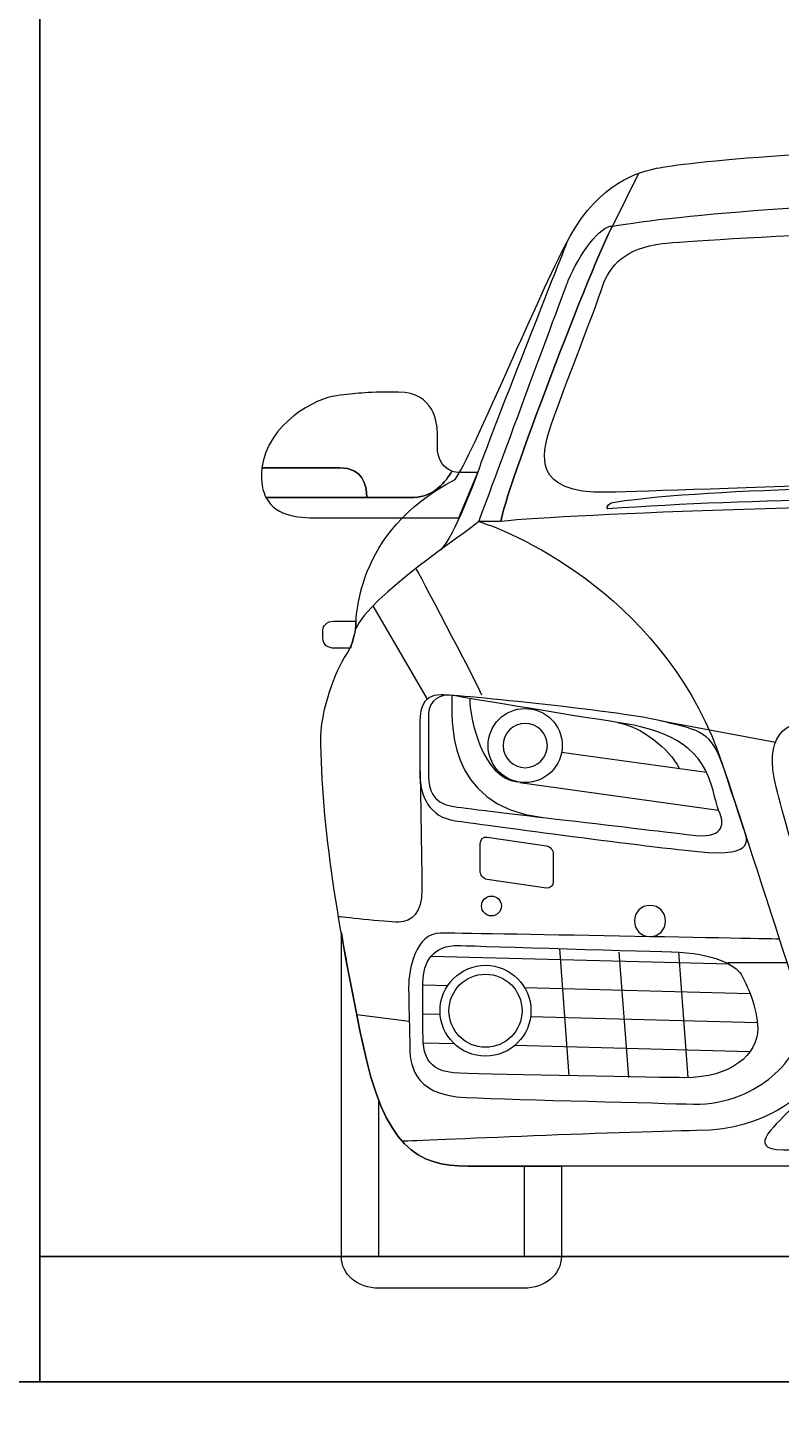
# Model space of a CAD drawing. Units: inches. Extents: x 1152 to 2588, y 1459 to 2618.
# Tile 9 of 17: x 1285 to 1321, y 2319 to 2386. Entities that reach past the tile are written whole.
import ezdxf

# ---------------------------------------------------------------- set-up
doc = ezdxf.new("R2010")
doc.units = ezdxf.units.IN
for name, color, linetype, lineweight in [('A-ANNO-DIMS', 2, 'Continuous', 18), ('A-ELEV', 7, 'Continuous', 25), ('AUDI', 7, 'Continuous', 13)]:
    doc.layers.add(name, color=color, linetype=linetype, lineweight=lineweight)
doc.styles.get("Standard").update_dxf_attribs({"font": 'arial.ttf'})
doc.dimstyles.get("Standard").update_dxf_attribs({"dimtxt": 0.18, "dimasz": 0.18, "dimexe": 0.18, "dimexo": 0.0625, "dimgap": 0.09, "dimtad": 0, "dimtih": 1, "dimtoh": 1, "dimdec": 4, "dimzin": 0, "dimdsep": 46, "dimtxsty": 'Standard', "dimcen": 0.09, "dimadec": 0, "dimazin": 0, "dimtfac": 1, "dimtdec": 4, "dimtofl": 0, "dimtmove": 0, "dimatfit": 3, "dimfxl": 1, "dimtolj": 1, "dimtzin": 0, "dimarcsym": 0})

# ---------------------------------------------------------------- blocks, each defined once
blk = doc.blocks.new('*D91')
at = {"layer": 'A-ANNO-DIMS', "color": 0, "lineweight": -2, "transparency": 16777216}
for p, q in [((1405.417, 2327.329), (1405.417, 2232.94)), ((1276.417, 2321.329), (1276.417, 2232.94)), ((1276.597, 2233.12), (1340.636, 2233.12)), ((1405.237, 2233.12), (1341.197, 2233.12))]:
    blk.add_line(p, q, dxfattribs=at)
at = {"layer": 'A-ANNO-DIMS', "color": 0, "transparency": 16777216}
for points in [[(1276.597, 2233.15), (1276.597, 2233.09), (1276.417, 2233.12)], [(1405.237, 2233.15), (1405.237, 2233.09), (1405.417, 2233.12)]]:
    blk.add_solid(points, dxfattribs=at)
at = {"layer": 'Defpoints', "color": 0, "transparency": 16777216}
for p in [(1405.417, 2327.391), (1276.417, 2321.391), (1405.417, 2233.12)]:
    blk.add_point(p, dxfattribs=at)
at = {"layer": 'A-ANNO-DIMS', "color": 0, "transparency": 16777216, "insert": (1340.917, 2233.12), "char_height": 0.18, "attachment_point": 5}
blk.add_mtext('\\A1;129', dxfattribs=at)

msp = doc.modelspace()

# ---------------------------------------------------------------- linework, layer by layer
at = {"layer": 'A-ELEV'}
for p, q in [((1285.4165, 2453.3911), (1285.4165, 2327.3911)), ((1736.4165, 2327.3911), (1285.4165, 2327.3911)), ((1285.4165, 2327.3911), (1285.4165, 2321.3911)), ((1736.4165, 2321.3911), (1276.4165, 2321.3911))]:
    msp.add_line(p, q, dxfattribs=at)
at = {"layer": 'AUDI'}
for points, knots in [([(1335.9514, 2380.6082), (1323.07, 2380.6082), (1316.2344, 2379.8209), (1314.9649, 2379.5565), (1314.9649, 2379.5565), (1313.6952, 2379.292), (1311.974, 2378.5979), (1310.5458, 2375.7943), (1310.5458, 2375.7943), (1309.1176, 2372.9909), (1306.1088, 2365.771), (1305.3217, 2364.6395), (1305.3217, 2364.6395), (1300.4024, 2362.1057), (1300.5918, 2357.8087), (1300.5428, 2357.4642), (1300.5428, 2357.4642), (1300.4936, 2357.1198), (1300.2995, 2356.5002), (1300.0824, 2356.2017), (1300.0824, 2356.2017), (1299.5785, 2355.5088), (1298.8858, 2353.5262), (1298.8858, 2352.3397), (1298.8858, 2352.3397), (1298.8858, 2347.9967), (1299.7554, 2343.0506), (1300.8566, 2337.73), (1300.8566, 2337.73), (1301.9224, 2332.5811), (1303.5104, 2331.7248), (1305.9177, 2331.7248), (1305.9177, 2331.7248), (1307.7191, 2331.725), (1335.9514, 2331.7248), (1335.9514, 2331.7248), (1335.9514, 2331.7248), (1335.9514, 2331.725), (1364.1837, 2331.7248), (1365.9852, 2331.7248), (1365.9852, 2331.7248), (1368.3925, 2331.725), (1369.9807, 2332.581), (1371.0466, 2337.73), (1371.0466, 2337.73), (1372.1483, 2343.0506), (1373.0181, 2347.9966), (1373.0181, 2352.3397), (1373.0181, 2352.3397), (1373.0181, 2353.5264), (1372.3251, 2355.5087), (1371.8212, 2356.2017), (1371.8212, 2356.2017), (1371.6039, 2356.5003), (1371.41, 2357.1198), (1371.3608, 2357.4642), (1371.3608, 2357.4642), (1371.3116, 2357.8087), (1371.501, 2362.1057), (1366.5811, 2364.6395), (1366.5811, 2364.6395), (1365.7941, 2365.7711), (1362.7853, 2372.9908), (1361.357, 2375.7943), (1361.357, 2375.7943), (1359.9288, 2378.5979), (1358.2076, 2379.292), (1356.9379, 2379.5565), (1356.9379, 2379.5565), (1355.6684, 2379.821), (1348.8329, 2380.608), (1335.9514, 2380.6082)], [0, 0, 0, 0, 0.0555556, 0.0555556, 0.0555556, 0.0555556, 0.1111111, 0.1111111, 0.1111111, 0.1111111, 0.1666667, 0.1666667, 0.1666667, 0.1666667, 0.2222222, 0.2222222, 0.2222222, 0.2222222, 0.2777778, 0.2777778, 0.2777778, 0.2777778, 0.3333333, 0.3333333, 0.3333333, 0.3333333, 0.3888889, 0.3888889, 0.3888889, 0.3888889, 0.4444444, 0.4444444, 0.4444444, 0.4444445, 0.5, 0.5, 0.5, 0.5, 0.5555556, 0.5555556, 0.5555556, 0.5555556, 0.6111111, 0.6111111, 0.6111111, 0.6111111, 0.6666667, 0.6666667, 0.6666667, 0.6666667, 0.7222222, 0.7222222, 0.7222222, 0.7222222, 0.7777778, 0.7777778, 0.7777778, 0.7777778, 0.8333333, 0.8333333, 0.8333333, 0.8333333, 0.8888889, 0.8888889, 0.8888889, 0.8888889, 0.9444444, 0.9444444, 0.9444444, 0.9444445, 1, 1, 1, 1]), ([(1335.9514, 2380.6082), (1323.07, 2380.6082), (1316.2344, 2379.8209), (1314.9649, 2379.5565), (1314.9649, 2379.5565), (1313.6952, 2379.292), (1311.974, 2378.5979), (1310.5458, 2375.7943), (1310.5458, 2375.7943), (1309.1176, 2372.9909), (1306.1088, 2365.771), (1305.3217, 2364.6395), (1305.3217, 2364.6395), (1300.4024, 2362.1057), (1300.5918, 2357.8087), (1300.5428, 2357.4642), (1300.5428, 2357.4642), (1300.4936, 2357.1198), (1300.2995, 2356.5002), (1300.0824, 2356.2017), (1300.0824, 2356.2017), (1299.5785, 2355.5088), (1298.8858, 2353.5262), (1298.8858, 2352.3397), (1298.8858, 2352.3397), (1298.8858, 2347.9967), (1299.7554, 2343.0506), (1300.8566, 2337.73), (1300.8566, 2337.73), (1301.9224, 2332.5811), (1303.5104, 2331.7248), (1305.9177, 2331.7248), (1305.9177, 2331.7248), (1307.7191, 2331.725), (1335.9514, 2331.7248), (1335.9514, 2331.7248), (1335.9514, 2331.7248), (1335.9514, 2331.7248), (1364.1837, 2331.7248), (1365.9852, 2331.7248), (1365.9852, 2331.7248), (1368.3925, 2331.725), (1369.9807, 2332.581), (1371.0466, 2337.73), (1371.0466, 2337.73), (1372.1483, 2343.0506), (1373.0181, 2347.9966), (1373.0181, 2352.3397), (1373.0181, 2352.3397), (1373.0181, 2353.5264), (1372.3251, 2355.5087), (1371.8212, 2356.2017), (1371.8212, 2356.2017), (1371.6039, 2356.5003), (1371.41, 2357.1198), (1371.3608, 2357.4642), (1371.3608, 2357.4642), (1371.3116, 2357.8087), (1371.501, 2362.1057), (1366.5811, 2364.6395), (1366.5811, 2364.6395), (1365.7941, 2365.7711), (1362.7853, 2372.9908), (1361.357, 2375.7943), (1361.357, 2375.7943), (1359.9288, 2378.5979), (1358.2076, 2379.292), (1356.9379, 2379.5565), (1356.9379, 2379.5565), (1355.6684, 2379.821), (1348.8329, 2380.608), (1335.9514, 2380.6082)], [0, 0, 0, 0, 0.0555556, 0.0555556, 0.0555556, 0.0555556, 0.1111111, 0.1111111, 0.1111111, 0.1111111, 0.1666667, 0.1666667, 0.1666667, 0.1666667, 0.2222222, 0.2222222, 0.2222222, 0.2222222, 0.2777778, 0.2777778, 0.2777778, 0.2777778, 0.3333333, 0.3333333, 0.3333333, 0.3333333, 0.3888889, 0.3888889, 0.3888889, 0.3888889, 0.4444444, 0.4444444, 0.4444444, 0.4444445, 0.5, 0.5, 0.5, 0.5, 0.5555556, 0.5555556, 0.5555556, 0.5555556, 0.6111111, 0.6111111, 0.6111111, 0.6111111, 0.6666667, 0.6666667, 0.6666667, 0.6666667, 0.7222222, 0.7222222, 0.7222222, 0.7222222, 0.7777778, 0.7777778, 0.7777778, 0.7777778, 0.8333333, 0.8333333, 0.8333333, 0.8333333, 0.8888889, 0.8888889, 0.8888889, 0.8888889, 0.9444444, 0.9444444, 0.9444444, 0.9444445, 1, 1, 1, 1]), ([(1335.9514, 2378.0831), (1323.862, 2378.0831), (1315.9013, 2377.3042), (1312.8453, 2376.7794), (1312.8453, 2376.7794), (1311.9763, 2375.2275), (1307.631, 2363.8673), (1307.5068, 2362.6256), (1307.5068, 2362.6256), (1310.8591, 2362.9982), (1325.7217, 2363.4947), (1335.9514, 2363.4947), (1335.9514, 2363.4947), (1346.1812, 2363.4947), (1361.0438, 2362.998), (1364.396, 2362.6256), (1364.396, 2362.6256), (1364.2719, 2363.8675), (1359.9266, 2375.2274), (1359.0575, 2376.7794), (1359.0575, 2376.7794), (1356.4376, 2377.3639), (1348.0408, 2378.0829), (1335.9514, 2378.0831)], [0, 0, 0, 0, 0.1666667, 0.1666667, 0.1666667, 0.1666667, 0.3333333, 0.3333333, 0.3333333, 0.3333333, 0.5, 0.5, 0.5, 0.5, 0.6666667, 0.6666667, 0.6666667, 0.6666667, 0.8333333, 0.8333333, 0.8333333, 0.8333333, 1, 1, 1, 1]), ([(1307.5069, 2362.6256), (1307.631, 2363.8675), (1311.9763, 2375.2274), (1312.8453, 2376.7794), (1312.8453, 2376.7794), (1312.2868, 2376.8414), (1311.2461, 2375.4309), (1310.7348, 2374.1721), (1310.7348, 2374.1721), (1310.5466, 2373.7086), (1306.4516, 2362.6256), (1306.4516, 2362.6256), (1306.4516, 2362.6256), (1306.4516, 2362.6256), (1307.5069, 2362.6256), (1307.5069, 2362.6256)], [0, 0, 0, 0, 0.25, 0.25, 0.25, 0.25, 0.5, 0.5, 0.5, 0.5, 0.75, 0.75, 0.75, 0.75, 1, 1, 1, 1]), ([(1335.9514, 2376.8669), (1331.6617, 2376.8669), (1317.0146, 2376.1677), (1315.2481, 2375.9467), (1315.2481, 2375.9467), (1313.4816, 2375.7259), (1312.7088, 2374.9163), (1312.3775, 2373.8859), (1312.3775, 2373.8859), (1312.0463, 2372.8554), (1310.1695, 2368.1078), (1309.8383, 2367.0037), (1309.8383, 2367.0037), (1309.5071, 2365.8998), (1308.9561, 2363.9401), (1312.5985, 2364.0229), (1312.5985, 2364.0229), (1316.4298, 2364.1101), (1333.6902, 2364.7958), (1335.9514, 2364.7958), (1335.9514, 2364.7958), (1338.2126, 2364.7959), (1355.473, 2364.1101), (1359.3043, 2364.0229), (1359.3043, 2364.0229), (1362.9467, 2363.9401), (1362.3958, 2365.8997), (1362.0646, 2367.0037), (1362.0646, 2367.0037), (1361.7334, 2368.1079), (1359.8565, 2372.8554), (1359.5253, 2373.8859), (1359.5253, 2373.8859), (1359.1941, 2374.9164), (1358.4212, 2375.7259), (1356.6547, 2375.9467), (1356.6547, 2375.9467), (1354.8882, 2376.1677), (1340.2411, 2376.8668), (1335.9514, 2376.8669)], [0, 0, 0, 0, 0.1, 0.1, 0.1, 0.1, 0.2, 0.2, 0.2, 0.2, 0.3, 0.3, 0.3, 0.3, 0.4, 0.4, 0.4, 0.4, 0.5, 0.5, 0.5, 0.5, 0.6, 0.6, 0.6, 0.6, 0.7, 0.7, 0.7, 0.7, 0.8, 0.8, 0.8, 0.8, 0.9, 0.9, 0.9, 0.9, 1, 1, 1, 1]), ([(1310.6985, 2376.0821), (1310.6985, 2376.0821), (1306.6845, 2365.9026), (1306.508, 2365.3031), (1306.508, 2365.3031), (1306.3315, 2364.7035), (1305.2287, 2361.8719), (1304.629, 2361.2722)], [0, 0, 0, 0, 0.5, 0.5, 0.5, 0.5, 1, 1, 1, 1]), ([(1299.7905, 2365.1973), (1298.8223, 2365.1973), (1297.0363, 2365.1973), (1296.0621, 2365.1973), (1296.0621, 2365.1973), (1296.323, 2367.3215), (1298.6669, 2368.5533), (1299.632, 2368.6531), (1299.632, 2368.6531), (1300.6547, 2368.759), (1300.8659, 2368.8293), (1302.5936, 2368.8293), (1302.5936, 2368.8293), (1304.3217, 2368.8294), (1304.4625, 2367.2778), (1304.4625, 2366.925), (1304.4625, 2366.925), (1304.4625, 2366.5723), (1304.4625, 2366.7135), (1304.4625, 2366.2552), (1304.4625, 2366.2552), (1304.4625, 2365.5383), (1304.7824, 2365.1733), (1305.1632, 2365.0364), (1305.1632, 2365.0364), (1304.8802, 2364.5611), (1304.3055, 2363.7821), (1303.3291, 2363.7821), (1303.3291, 2363.7821), (1302.9462, 2363.7822), (1302.0943, 2363.7821), (1301.0908, 2363.7821), (1301.0908, 2363.7821), (1301.0651, 2364.3736), (1300.8906, 2365.1973), (1299.7905, 2365.1973)], [0, 0, 0, 0, 0.1111111, 0.1111111, 0.1111111, 0.1111111, 0.2222222, 0.2222222, 0.2222222, 0.2222222, 0.3333333, 0.3333333, 0.3333333, 0.3333333, 0.4444444, 0.4444444, 0.4444444, 0.4444445, 0.5555556, 0.5555556, 0.5555556, 0.5555556, 0.6666667, 0.6666667, 0.6666667, 0.6666667, 0.7777778, 0.7777778, 0.7777778, 0.7777778, 0.8888889, 0.8888889, 0.8888889, 0.8888889, 1, 1, 1, 1]), ([(1299.7905, 2365.1973), (1300.8906, 2365.1973), (1301.0651, 2364.3735), (1301.0908, 2363.7821), (1301.0908, 2363.7821), (1299.405, 2363.7822), (1297.291, 2363.7821), (1296.2512, 2363.7821), (1296.2512, 2363.7821), (1296.1175, 2364.0477), (1296.0358, 2364.3803), (1296.0358, 2364.8092), (1296.0358, 2364.8092), (1296.0358, 2364.9422), (1296.0466, 2365.0706), (1296.0621, 2365.1973), (1296.0621, 2365.1973), (1297.0364, 2365.1973), (1298.8223, 2365.1973), (1299.7905, 2365.1973)], [0, 0, 0, 0, 0.2, 0.2, 0.2, 0.2, 0.4, 0.4, 0.4, 0.4, 0.6, 0.6, 0.6, 0.6, 0.8, 0.8, 0.8, 0.8, 1, 1, 1, 1]), ([(1303.3291, 2363.7822), (1304.3055, 2363.7822), (1304.8802, 2364.561), (1305.1632, 2365.0364), (1305.1632, 2365.0364), (1305.2882, 2364.9918), (1305.4194, 2364.9709), (1305.5483, 2364.9709), (1305.5483, 2364.9709), (1306.0699, 2364.971), (1306.4022, 2364.9709), (1306.4022, 2364.9709), (1306.4022, 2364.9709), (1306.4022, 2364.9709), (1305.4953, 2362.7992), (1305.4953, 2362.7992), (1305.4953, 2362.7992), (1305.4953, 2362.7992), (1300.0197, 2362.7991), (1298.8858, 2362.7991), (1298.8858, 2362.7991), (1297.9935, 2362.7992), (1296.7448, 2362.8035), (1296.2512, 2363.7821), (1296.2512, 2363.7821), (1297.9098, 2363.7822), (1302.3028, 2363.7821), (1303.3291, 2363.7822)], [0, 0, 0, 0, 0.1428571, 0.1428571, 0.1428571, 0.1428572, 0.2857143, 0.2857143, 0.2857143, 0.2857143, 0.4285714, 0.4285714, 0.4285714, 0.4285714, 0.5714286, 0.5714286, 0.5714286, 0.5714286, 0.7142857, 0.7142857, 0.7142857, 0.7142857, 0.8571429, 0.8571429, 0.8571429, 0.8571429, 1, 1, 1, 1]), ([(1333.7843, 2364.2972), (1327.6294, 2364.315), (1317.9085, 2364.2868), (1312.9628, 2363.5578), (1312.9628, 2363.5578), (1312.7186, 2363.5304), (1312.5333, 2363.3499), (1312.6234, 2363.227), (1312.6234, 2363.227), (1319.8823, 2363.7437), (1327.6218, 2363.7359), (1335.1175, 2363.7009), (1335.1175, 2363.7009), (1334.9378, 2363.9473), (1334.4852, 2364.288), (1333.7843, 2364.2972)], [0, 0, 0, 0, 0.25, 0.25, 0.25, 0.25, 0.5, 0.5, 0.5, 0.5, 0.75, 0.75, 0.75, 0.75, 1, 1, 1, 1]), ([(1333.7843, 2364.2972), (1327.6294, 2364.315), (1317.9085, 2364.2868), (1312.9628, 2363.5578), (1312.9628, 2363.5578), (1312.7186, 2363.5304), (1312.5333, 2363.3499), (1312.6234, 2363.227), (1312.6234, 2363.227), (1319.8823, 2363.7437), (1327.6218, 2363.7359), (1335.1175, 2363.7009), (1335.1175, 2363.7009), (1334.9378, 2363.9473), (1334.4852, 2364.288), (1333.7843, 2364.2972)], [0, 0, 0, 0, 0.25, 0.25, 0.25, 0.25, 0.5, 0.5, 0.5, 0.5, 0.75, 0.75, 0.75, 0.75, 1, 1, 1, 1]), ([(1333.7843, 2364.2972), (1327.6294, 2364.315), (1317.9085, 2364.2868), (1312.9628, 2363.5578), (1312.9628, 2363.5578), (1312.7186, 2363.5304), (1312.5333, 2363.3499), (1312.6234, 2363.227), (1312.6234, 2363.227), (1319.8823, 2363.7437), (1327.6218, 2363.7359), (1335.1175, 2363.7009), (1335.1175, 2363.7009), (1334.9378, 2363.9473), (1334.4852, 2364.288), (1333.7843, 2364.2972)], [0, 0, 0, 0, 0.25, 0.25, 0.25, 0.25, 0.5, 0.5, 0.5, 0.5, 0.75, 0.75, 0.75, 0.75, 1, 1, 1, 1]), ([(1306.4516, 2362.6256), (1308.2711, 2362.0587), (1315.536, 2358.8847), (1318.1455, 2350.9148), (1318.1455, 2350.9148), (1320.7551, 2342.9449), (1323.0393, 2335.7729), (1323.0393, 2335.7729)], [0, 0, 0, 0, 0.5, 0.5, 0.5, 0.5, 1, 1, 1, 1]), ([(1300.5654, 2357.8463), (1300.5654, 2357.8463), (1299.7848, 2357.8463), (1299.4804, 2357.8463), (1299.4804, 2357.8463), (1299.1761, 2357.8463), (1298.9777, 2357.6221), (1298.9777, 2357.4235), (1298.9777, 2357.4235), (1298.9777, 2357.225), (1298.9777, 2357.4132), (1298.9777, 2357.0433), (1298.9777, 2357.0433), (1298.9777, 2356.708), (1299.2267, 2356.5507), (1299.5445, 2356.5507), (1299.5445, 2356.5507), (1299.8622, 2356.5508), (1300.3001, 2356.5562), (1300.3001, 2356.5562), (1300.3001, 2356.5562), (1300.3001, 2356.5564), (1300.565, 2357.2497), (1300.5654, 2357.8463)], [0, 0, 0, 0, 0.1666667, 0.1666667, 0.1666667, 0.1666667, 0.3333333, 0.3333333, 0.3333333, 0.3333333, 0.5, 0.5, 0.5, 0.5, 0.6666667, 0.6666667, 0.6666667, 0.6666667, 0.8333333, 0.8333333, 0.8333333, 0.8333333, 1, 1, 1, 1]), ([(1300.5654, 2357.8463), (1300.5654, 2357.8463), (1299.7848, 2357.8463), (1299.4804, 2357.8463), (1299.4804, 2357.8463), (1299.1761, 2357.8463), (1298.9777, 2357.6221), (1298.9777, 2357.4235), (1298.9777, 2357.4235), (1298.9777, 2357.225), (1298.9777, 2357.4132), (1298.9777, 2357.0433), (1298.9777, 2357.0433), (1298.9777, 2356.708), (1299.2267, 2356.5507), (1299.5445, 2356.5507), (1299.5445, 2356.5507), (1299.8622, 2356.5508), (1300.3001, 2356.5562), (1300.3001, 2356.5562), (1300.3001, 2356.5562), (1300.3001, 2356.5562), (1300.5654, 2357.2497), (1300.5654, 2357.8463)], [0, 0, 0, 0, 0.1666667, 0.1666667, 0.1666667, 0.1666667, 0.3333333, 0.3333333, 0.3333333, 0.3333333, 0.5, 0.5, 0.5, 0.5, 0.6666667, 0.6666667, 0.6666667, 0.6666667, 0.8333333, 0.8333333, 0.8333333, 0.8333333, 1, 1, 1, 1]), ([(1304.6531, 2354.3162), (1305.4033, 2354.3162), (1313.6008, 2353.5024), (1315.3347, 2353.0315), (1315.3347, 2353.0315), (1317.0686, 2352.5608), (1317.5822, 2352.6395), (1318.2128, 2350.7088), (1318.2128, 2350.7088), (1318.8435, 2348.7781), (1318.9129, 2348.5655), (1319.0908, 2348.0188), (1319.0908, 2348.0188), (1319.2688, 2347.4722), (1319.894, 2346.5027), (1316.94, 2346.8024), (1316.94, 2346.8024), (1313.986, 2347.102), (1306.5367, 2348.1084), (1305.3165, 2348.2794), (1305.3165, 2348.2794), (1304.0964, 2348.4506), (1303.6254, 2349.4353), (1303.6254, 2350.5484), (1303.6254, 2350.5484), (1303.6254, 2351.6615), (1303.6254, 2352.175), (1303.6254, 2352.7959), (1303.6254, 2352.7959), (1303.6254, 2353.4171), (1303.6043, 2354.3159), (1304.6531, 2354.3162)], [0, 0, 0, 0, 0.125, 0.125, 0.125, 0.125, 0.25, 0.25, 0.25, 0.25, 0.375, 0.375, 0.375, 0.375, 0.5, 0.5, 0.5, 0.5, 0.625, 0.625, 0.625, 0.625, 0.75, 0.75, 0.75, 0.75, 0.875, 0.875, 0.875, 0.875, 1, 1, 1, 1]), ([(1305.1636, 2354.2871), (1305.1636, 2354.2871), (1310.9161, 2353.3127), (1313.0849, 2352.9953), (1313.0849, 2352.9953), (1315.2537, 2352.6781), (1316.9993, 2351.9903), (1317.5811, 2350.0331), (1317.5811, 2350.0331), (1317.8456, 2349.134), (1317.7927, 2349.1338), (1318.0043, 2348.6049), (1318.0043, 2348.6049), (1318.216, 2348.0759), (1318.1631, 2347.3881), (1316.5761, 2347.5998), (1316.5761, 2347.5998), (1314.9892, 2347.8115), (1306.0993, 2348.8166), (1305.1502, 2348.9752), (1305.1502, 2348.9752), (1304.2239, 2349.1299), (1304.0394, 2349.8403), (1304.0394, 2350.3693), (1304.0394, 2350.3693), (1304.0394, 2350.8983), (1304.0394, 2352.7796), (1304.0394, 2353.4185), (1304.0394, 2353.4185), (1304.0394, 2354.0577), (1304.6501, 2354.3736), (1305.1636, 2354.2871)], [0, 0, 0, 0, 0.125, 0.125, 0.125, 0.125, 0.25, 0.25, 0.25, 0.25, 0.375, 0.375, 0.375, 0.375, 0.5, 0.5, 0.5, 0.5, 0.625, 0.625, 0.625, 0.625, 0.75, 0.75, 0.75, 0.75, 0.875, 0.875, 0.875, 0.875, 1, 1, 1, 1]), ([(1310.4462, 2351.8838), (1310.4462, 2352.8648), (1309.651, 2353.6599), (1308.67, 2353.6599), (1308.67, 2353.6599), (1307.6889, 2353.6601), (1306.8935, 2352.8648), (1306.8935, 2351.8837), (1306.8935, 2351.8837), (1306.8935, 2350.9027), (1307.6889, 2350.1072), (1308.67, 2350.1072), (1308.67, 2350.1072), (1309.651, 2350.1073), (1310.4462, 2350.9025), (1310.4462, 2351.8838)], [0, 0, 0, 0, 0.25, 0.25, 0.25, 0.25, 0.5, 0.5, 0.5, 0.5, 0.75, 0.75, 0.75, 0.75, 1, 1, 1, 1]), ([(1307.6073, 2351.8838), (1307.6073, 2352.4706), (1308.0829, 2352.9461), (1308.67, 2352.9461), (1308.67, 2352.9461), (1309.2568, 2352.9463), (1309.7325, 2352.4705), (1309.7325, 2351.8837), (1309.7325, 2351.8837), (1309.7325, 2351.2966), (1309.2568, 2350.821), (1308.67, 2350.821), (1308.67, 2350.821), (1308.0829, 2350.821), (1307.6073, 2351.2966), (1307.6073, 2351.8838)], [0, 0, 0, 0, 0.25, 0.25, 0.25, 0.25, 0.5, 0.5, 0.5, 0.5, 0.75, 0.75, 0.75, 0.75, 1, 1, 1, 1]), ([(1335.9514, 2353.4829), (1334.637, 2353.4829), (1324.1786, 2353.3822), (1322.6342, 2353.2057), (1322.6342, 2353.2057), (1321.0898, 2353.0293), (1320.0748, 2352.3234), (1320.6926, 2349.8963), (1320.6926, 2349.8963), (1321.3105, 2347.4694), (1323.3842, 2340.3645), (1323.7374, 2339.2174), (1323.7374, 2339.2174), (1324.0905, 2338.0701), (1324.5802, 2337.1609), (1327.1353, 2337.0109), (1327.1353, 2337.0109), (1328.6449, 2336.9224), (1333.7102, 2336.8908), (1335.9514, 2336.8908), (1335.9514, 2336.8908), (1338.1926, 2336.8909), (1343.2579, 2336.9224), (1344.7675, 2337.0109), (1344.7675, 2337.0109), (1347.3226, 2337.1611), (1347.8123, 2338.0701), (1348.1655, 2339.2174), (1348.1655, 2339.2174), (1348.5186, 2340.3646), (1350.5923, 2347.4691), (1351.2102, 2349.8963), (1351.2102, 2349.8963), (1351.828, 2352.3236), (1350.813, 2353.0293), (1349.2687, 2353.2057), (1349.2687, 2353.2057), (1347.7244, 2353.3823), (1337.2658, 2353.4828), (1335.9514, 2353.4829)], [0, 0, 0, 0, 0.1, 0.1, 0.1, 0.1, 0.2, 0.2, 0.2, 0.2, 0.3, 0.3, 0.3, 0.3, 0.4, 0.4, 0.4, 0.4, 0.5, 0.5, 0.5, 0.5, 0.6, 0.6, 0.6, 0.6, 0.7, 0.7, 0.7, 0.7, 0.8, 0.8, 0.8, 0.8, 0.9, 0.9, 0.9, 0.9, 1, 1, 1, 1]), ([(1303.6254, 2351.0383), (1303.6254, 2351.0383), (1303.722, 2346.0128), (1303.722, 2344.9549), (1303.722, 2344.9549), (1303.722, 2343.8971), (1303.2459, 2343.4208), (1302.6111, 2343.4208), (1302.6111, 2343.4208), (1301.9766, 2343.421), (1299.7269, 2343.6806), (1299.7269, 2343.6806)], [0, 0, 0, 0, 0.3333333, 0.3333333, 0.3333333, 0.3333333, 0.6666667, 0.6666667, 0.6666667, 0.6666667, 1, 1, 1, 1]), ([(1306.5117, 2345.8748), (1306.5117, 2345.6736), (1306.6596, 2345.489), (1306.8426, 2345.4624), (1306.8426, 2345.4624), (1306.8426, 2345.4624), (1309.6849, 2345.048), (1309.6849, 2345.048), (1309.6849, 2345.048), (1309.8678, 2345.0214), (1310.0164, 2345.1626), (1310.0164, 2345.3636), (1310.0164, 2345.3636), (1310.0164, 2345.3636), (1310.0176, 2346.6682), (1310.0176, 2346.6682), (1310.0176, 2346.6682), (1310.0176, 2346.8693), (1309.8694, 2347.0536), (1309.6866, 2347.0803), (1309.6866, 2347.0803), (1309.6866, 2347.0803), (1306.8441, 2347.4949), (1306.8441, 2347.4949), (1306.8441, 2347.4949), (1306.6613, 2347.5215), (1306.5127, 2347.3801), (1306.5127, 2347.1791), (1306.5127, 2347.1791), (1306.5127, 2347.1791), (1306.5117, 2345.8748), (1306.5117, 2345.8748)], [0, 0, 0, 0, 0.125, 0.125, 0.125, 0.125, 0.25, 0.25, 0.25, 0.25, 0.375, 0.375, 0.375, 0.375, 0.5, 0.5, 0.5, 0.5, 0.625, 0.625, 0.625, 0.625, 0.75, 0.75, 0.75, 0.75, 0.875, 0.875, 0.875, 0.875, 1, 1, 1, 1]), ([(1307.5306, 2344.1942), (1307.5306, 2344.457), (1307.3174, 2344.6702), (1307.0545, 2344.6702), (1307.0545, 2344.6702), (1306.7917, 2344.6703), (1306.5784, 2344.4569), (1306.5784, 2344.194), (1306.5784, 2344.194), (1306.5784, 2343.9313), (1306.7917, 2343.7179), (1307.0545, 2343.7179), (1307.0545, 2343.7179), (1307.3174, 2343.7181), (1307.5306, 2343.9312), (1307.5306, 2344.1942)], [0, 0, 0, 0, 0.25, 0.25, 0.25, 0.25, 0.5, 0.5, 0.5, 0.5, 0.75, 0.75, 0.75, 0.75, 1, 1, 1, 1]), ([(1313.9002, 2343.4738), (1313.9002, 2343.8871), (1314.2352, 2344.2218), (1314.6482, 2344.2218), (1314.6482, 2344.2218), (1315.0613, 2344.2218), (1315.3962, 2343.8871), (1315.3962, 2343.4737), (1315.3962, 2343.4737), (1315.3962, 2343.0607), (1315.0613, 2342.7258), (1314.6482, 2342.7258), (1314.6482, 2342.7258), (1314.2352, 2342.726), (1313.9002, 2343.0604), (1313.9002, 2343.4738)], [0, 0, 0, 0, 0.25, 0.25, 0.25, 0.25, 0.5, 0.5, 0.5, 0.5, 0.75, 0.75, 0.75, 0.75, 1, 1, 1, 1]), ([(1300.8566, 2337.73), (1300.4906, 2339.4986), (1300.1547, 2341.221), (1299.8633, 2342.8986), (1299.8633, 2342.8986), (1299.8633, 2342.8986), (1299.8633, 2327.3911), (1299.8633, 2327.3911), (1299.8633, 2327.3911), (1299.8633, 2326.5378), (1300.6429, 2325.8678), (1301.6592, 2325.8678), (1301.6592, 2325.8678), (1301.6592, 2325.8678), (1308.608, 2325.8679), (1308.608, 2325.8679), (1308.608, 2325.8679), (1309.6246, 2325.8679), (1310.4045, 2326.5378), (1310.4045, 2327.3909), (1310.4045, 2327.3909), (1310.4045, 2327.3909), (1310.4045, 2331.725), (1310.4045, 2331.725), (1310.4045, 2331.725), (1308.0102, 2331.725), (1306.3162, 2331.7248), (1305.9177, 2331.7248), (1305.9177, 2331.7248), (1303.5104, 2331.725), (1301.9224, 2332.581), (1300.8566, 2337.73)], [0, 0, 0, 0, 0.125, 0.125, 0.125, 0.125, 0.25, 0.25, 0.25, 0.25, 0.375, 0.375, 0.375, 0.375, 0.5, 0.5, 0.5, 0.5, 0.625, 0.625, 0.625, 0.625, 0.75, 0.75, 0.75, 0.75, 0.875, 0.875, 0.875, 0.875, 1, 1, 1, 1]), ([(1320.8458, 2342.6054), (1320.8458, 2342.6054), (1305.8379, 2342.8919), (1304.6212, 2342.8919), (1304.6212, 2342.8919), (1303.4046, 2342.8919), (1303.0872, 2341.1463), (1303.0872, 2340.2999), (1303.0872, 2340.2999), (1303.0872, 2339.4536), (1303.1401, 2338.2368), (1303.1401, 2337.4963), (1303.1401, 2337.4963), (1303.1401, 2336.7559), (1303.193, 2335.1159), (1305.8379, 2335.0101), (1305.8379, 2335.0101), (1308.4827, 2334.9044), (1315.1479, 2334.7456), (1316.7348, 2334.6927), (1316.7348, 2334.6927), (1318.3218, 2334.6399), (1319.75, 2335.3804), (1320.4906, 2336.0151), (1320.4906, 2336.0151), (1321.2312, 2336.6499), (1322.3377, 2337.9711), (1321.8613, 2339.452)], [0, 0, 0, 0, 0.1428571, 0.1428571, 0.1428571, 0.1428572, 0.2857143, 0.2857143, 0.2857143, 0.2857143, 0.4285714, 0.4285714, 0.4285714, 0.4285714, 0.5714286, 0.5714286, 0.5714286, 0.5714286, 0.7142857, 0.7142857, 0.7142857, 0.7142857, 0.8571429, 0.8571429, 0.8571429, 0.8571429, 1, 1, 1, 1]), ([(1305.4924, 2342.2994), (1304.241, 2342.3251), (1303.7749, 2341.5165), (1303.7749, 2340.5115), (1303.7749, 2340.5115), (1303.7749, 2339.5065), (1303.7749, 2339.0304), (1303.7749, 2338.131), (1303.7749, 2338.131), (1303.7749, 2337.232), (1303.8278, 2336.2267), (1305.5205, 2336.1738), (1305.5205, 2336.1738), (1307.2132, 2336.121), (1315.3595, 2335.9622), (1316.3116, 2335.9622), (1316.3116, 2335.9622), (1318.5323, 2335.9623), (1319.8089, 2337.0692), (1319.8089, 2338.3206), (1319.8089, 2338.3206), (1319.8089, 2339.2729), (1319.2725, 2340.5003), (1319.008, 2340.9235), (1319.008, 2340.9235), (1318.7435, 2341.3467), (1317.7398, 2341.9397), (1315.6768, 2341.9926), (1315.6768, 2341.9926), (1313.6139, 2342.0456), (1305.4924, 2342.2992), (1305.4924, 2342.2994)], [0, 0, 0, 0, 0.125, 0.125, 0.125, 0.125, 0.25, 0.25, 0.25, 0.25, 0.375, 0.375, 0.375, 0.375, 0.5, 0.5, 0.5, 0.5, 0.625, 0.625, 0.625, 0.625, 0.75, 0.75, 0.75, 0.75, 0.875, 0.875, 0.875, 0.875, 1, 1, 1, 1]), ([(1305.4924, 2342.2994), (1304.241, 2342.3251), (1303.7749, 2341.5165), (1303.7749, 2340.5115), (1303.7749, 2340.5115), (1303.7749, 2339.5065), (1303.7749, 2339.0304), (1303.7749, 2338.131), (1303.7749, 2338.131), (1303.7749, 2337.232), (1303.8278, 2336.2267), (1305.5205, 2336.1738), (1305.5205, 2336.1738), (1307.2132, 2336.121), (1315.3595, 2335.9622), (1316.3116, 2335.9622), (1316.3116, 2335.9622), (1318.5323, 2335.9623), (1319.8089, 2337.0692), (1319.8089, 2338.3206), (1319.8089, 2338.3206), (1319.8089, 2339.2729), (1319.2725, 2340.5003), (1319.008, 2340.9235), (1319.008, 2340.9235), (1318.7435, 2341.3467), (1317.7398, 2341.9397), (1315.6768, 2341.9926), (1315.6768, 2341.9926), (1313.6139, 2342.0456), (1305.4924, 2342.2994), (1305.4924, 2342.2994)], [0, 0, 0, 0, 0.125, 0.125, 0.125, 0.125, 0.25, 0.25, 0.25, 0.25, 0.375, 0.375, 0.375, 0.375, 0.5, 0.5, 0.5, 0.5, 0.625, 0.625, 0.625, 0.625, 0.75, 0.75, 0.75, 0.75, 0.875, 0.875, 0.875, 0.875, 1, 1, 1, 1]), ([(1308.9465, 2339.1716), (1308.9465, 2340.3741), (1307.9716, 2341.3489), (1306.7689, 2341.3489), (1306.7689, 2341.3489), (1305.5663, 2341.3491), (1304.5914, 2340.374), (1304.5914, 2339.1714), (1304.5914, 2339.1714), (1304.5914, 2337.969), (1305.5663, 2336.994), (1306.7689, 2336.994), (1306.7689, 2336.994), (1307.9716, 2336.9942), (1308.9465, 2337.9689), (1308.9465, 2339.1716)], [0, 0, 0, 0, 0.25, 0.25, 0.25, 0.25, 0.5, 0.5, 0.5, 0.5, 0.75, 0.75, 0.75, 0.75, 1, 1, 1, 1]), ([(1308.5193, 2339.1716), (1308.5193, 2340.1384), (1307.7356, 2340.9218), (1306.7689, 2340.9218), (1306.7689, 2340.9218), (1305.8023, 2340.9218), (1305.0185, 2340.1383), (1305.0185, 2339.1714), (1305.0185, 2339.1714), (1305.0185, 2338.2046), (1305.8023, 2337.4211), (1306.7689, 2337.4211), (1306.7689, 2337.4211), (1307.7356, 2337.4213), (1308.5193, 2338.2046), (1308.5193, 2339.1716)], [0, 0, 0, 0, 0.25, 0.25, 0.25, 0.25, 0.5, 0.5, 0.5, 0.5, 0.75, 0.75, 0.75, 0.75, 1, 1, 1, 1]), ([(1335.9514, 2332.5064), (1335.9514, 2332.5064), (1323.0118, 2332.5064), (1321.0371, 2332.5064), (1321.0371, 2332.5064), (1319.0624, 2332.5064), (1320.896, 2333.8463), (1321.4603, 2334.5515), (1321.4603, 2334.5515), (1322.0246, 2335.257), (1323.0693, 2336.2444), (1325.6922, 2336.2444), (1325.6922, 2336.2444), (1328.3149, 2336.2444), (1335.9514, 2336.2444), (1335.9514, 2336.2444), (1335.9514, 2336.2444), (1335.9514, 2336.2444), (1343.5879, 2336.2444), (1346.2106, 2336.2444), (1346.2106, 2336.2444), (1348.8335, 2336.2444), (1349.8782, 2335.2569), (1350.4425, 2334.5515), (1350.4425, 2334.5515), (1351.0069, 2333.8463), (1352.8404, 2332.5064), (1350.8657, 2332.5064), (1350.8657, 2332.5064), (1348.891, 2332.5064), (1335.9514, 2332.5064), (1335.9514, 2332.5064)], [0, 0, 0, 0, 0.125, 0.125, 0.125, 0.125, 0.25, 0.25, 0.25, 0.25, 0.375, 0.375, 0.375, 0.375, 0.5, 0.5, 0.5, 0.5, 0.625, 0.625, 0.625, 0.625, 0.75, 0.75, 0.75, 0.75, 0.875, 0.875, 0.875, 0.875, 1, 1, 1, 1]), ([(1322.7487, 2335.6318), (1321.6014, 2335.2217), (1320.4906, 2333.4761), (1316.8935, 2333.4232), (1316.8935, 2333.4232), (1313.2965, 2333.3703), (1302.7789, 2332.9116), (1302.7789, 2332.9116)], [0, 0, 0, 0, 0.5, 0.5, 0.5, 0.5, 1, 1, 1, 1])]:
    msp.add_open_spline(points, degree=3, knots=knots, dxfattribs=at)
for points in [[(1314.0913, 2379.308), (1314.0913, 2379.308), (1312.8453, 2376.7795), (1312.8453, 2376.7795)], [(1306.4516, 2362.6256), (1305.8732, 2362.0938), (1301.2068, 2359.058), (1300.5428, 2357.4642)], [(1303.4385, 2360.3723), (1303.4385, 2360.3723), (1306.2081, 2355.1641), (1306.5784, 2354.3178)], [(1301.3696, 2358.5742), (1301.3696, 2358.5742), (1303.9816, 2354.1126), (1303.9816, 2354.1126)], [(1305.1636, 2354.2871), (1305.1636, 2353.2599), (1304.745, 2348.9973), (1309.5271, 2348.4362)], [(1306.0119, 2354.1443), (1306.0119, 2353.2072), (1306.6094, 2350.3368), (1308.2794, 2350.1515)], [(1313.0849, 2352.9954), (1314.2414, 2352.7751), (1315.5657, 2351.7638), (1316.0445, 2350.7927)], [(1315.1183, 2353.0848), (1315.1183, 2353.0848), (1320.661, 2352.0479), (1320.661, 2352.0479)], [(1310.4164, 2351.5677), (1310.4164, 2351.5677), (1317.3545, 2350.6122), (1317.3545, 2350.6122)], [(1308.4189, 2350.1073), (1308.4189, 2350.1073), (1317.9337, 2348.7882), (1317.9337, 2348.7882)], [(1318.4495, 2341.397), (1318.4495, 2341.397), (1304.1528, 2341.7769), (1304.1528, 2341.7769)], [(1310.3164, 2342.1503), (1310.3164, 2342.1503), (1310.7611, 2336.0567), (1310.7611, 2336.0567)], [(1313.163, 2341.979), (1313.163, 2341.979), (1313.612, 2335.9649), (1313.612, 2335.9649)], [(1316.0073, 2341.979), (1316.0073, 2341.979), (1316.4563, 2335.9649), (1316.4563, 2335.9649)], [(1318.3844, 2341.4908), (1318.3844, 2341.4908), (1321.1857, 2341.4908), (1321.1857, 2341.4908)], [(1304.9498, 2340.3676), (1304.9498, 2340.3676), (1303.791, 2340.3984), (1303.791, 2340.3984)], [(1319.4348, 2339.9823), (1319.4348, 2339.9823), (1308.6489, 2340.2694), (1308.6489, 2340.2694)], [(1303.1188, 2338.6623), (1303.1188, 2338.6623), (1300.6018, 2338.9776), (1300.6018, 2338.9776)], [(1304.5994, 2338.989), (1304.5994, 2338.989), (1303.791, 2339.0098), (1303.791, 2339.0098)], [(1319.7963, 2338.5941), (1319.7963, 2338.5941), (1308.9256, 2338.8766), (1308.9256, 2338.8766)], [(1305.2835, 2337.5819), (1305.2835, 2337.5819), (1303.791, 2337.6217), (1303.791, 2337.6217)], [(1319.4348, 2337.2056), (1319.4348, 2337.2056), (1308.1701, 2337.505), (1308.1701, 2337.505)], [(1301.6592, 2327.3911), (1301.6592, 2327.3911), (1301.6592, 2334.8073), (1301.6592, 2334.8073)], [(1308.6417, 2327.3911), (1308.6417, 2327.3911), (1308.6417, 2331.725), (1308.6417, 2331.725)]]:
    msp.add_open_spline(points, degree=3, dxfattribs=at)

# ---------------------------------------------------------------- dimensions: what is measured, and where the dimension line sits
at = {"layer": 'A-ANNO-DIMS'}
dim = msp.add_linear_dim(base=(1405.4165, 2233.12), p1=(1276.4165, 2321.3911), p2=(1405.4165, 2327.3911), dimstyle='Standard', override={"dimdec": 0, "dimlfac": 1, "dimrnd": 0, "dimzin": 0, "dimdsep": 46, "dimlunit": 2}, dxfattribs=at)
dim.commit()
dim.dimension.update_dxf_attribs({"geometry": '*D91', "text_midpoint": (1340.9165, 2233.12)})

doc.saveas('drawing.dxf')
